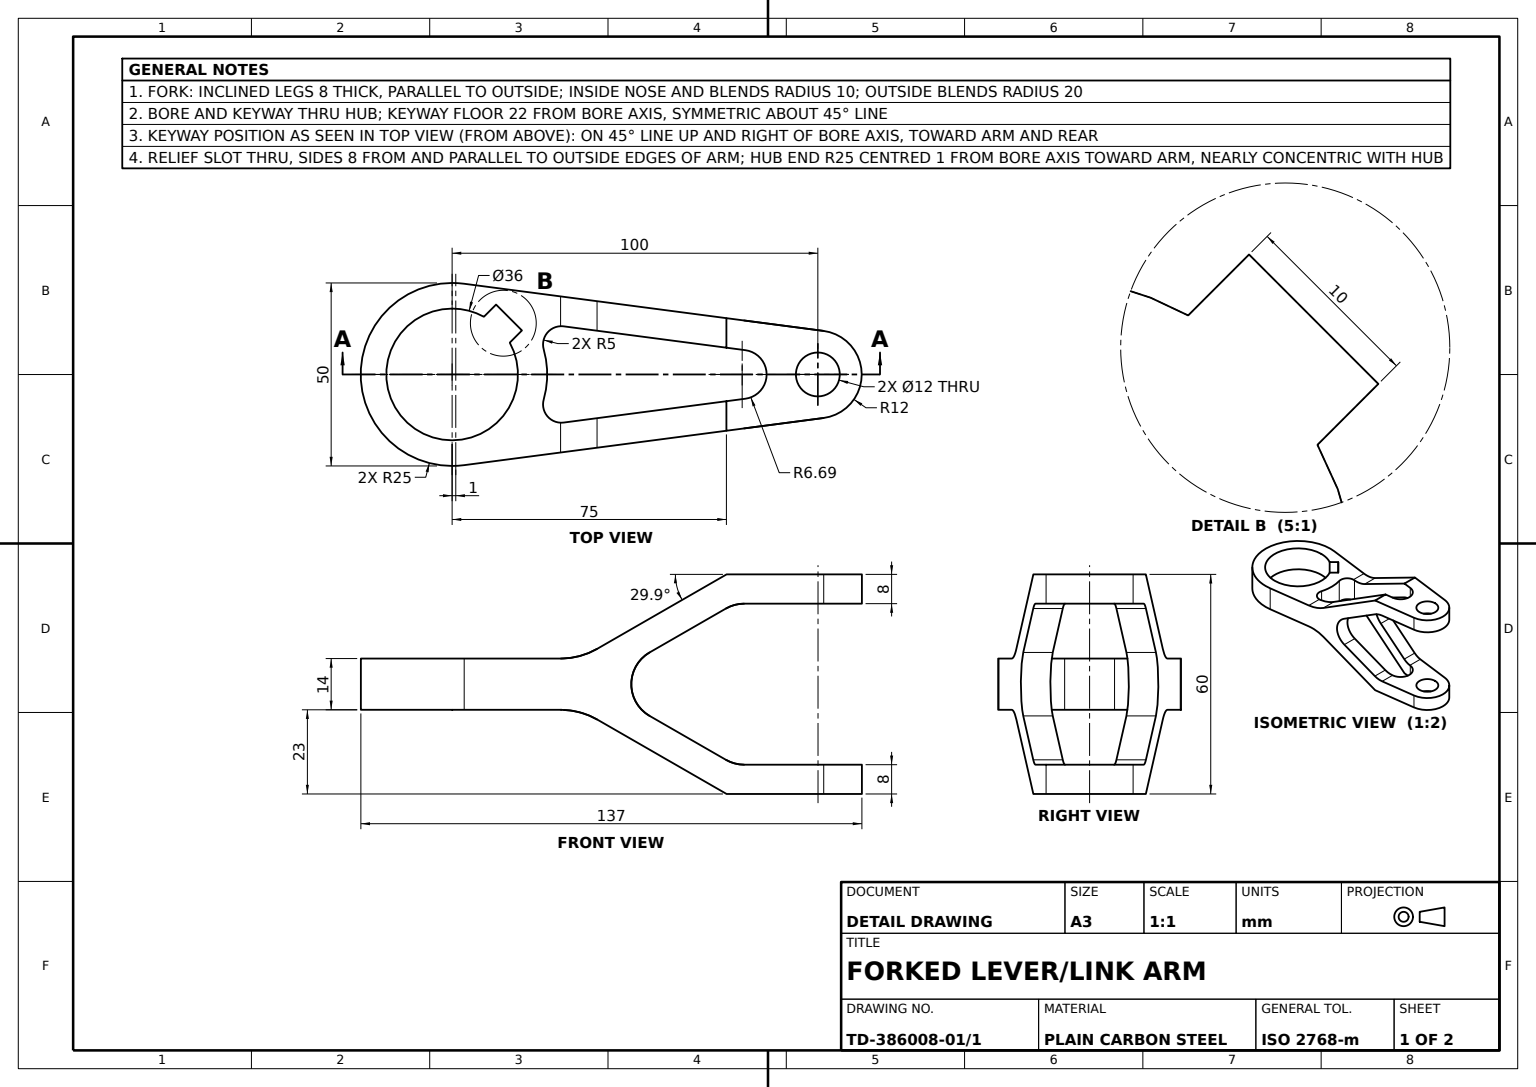
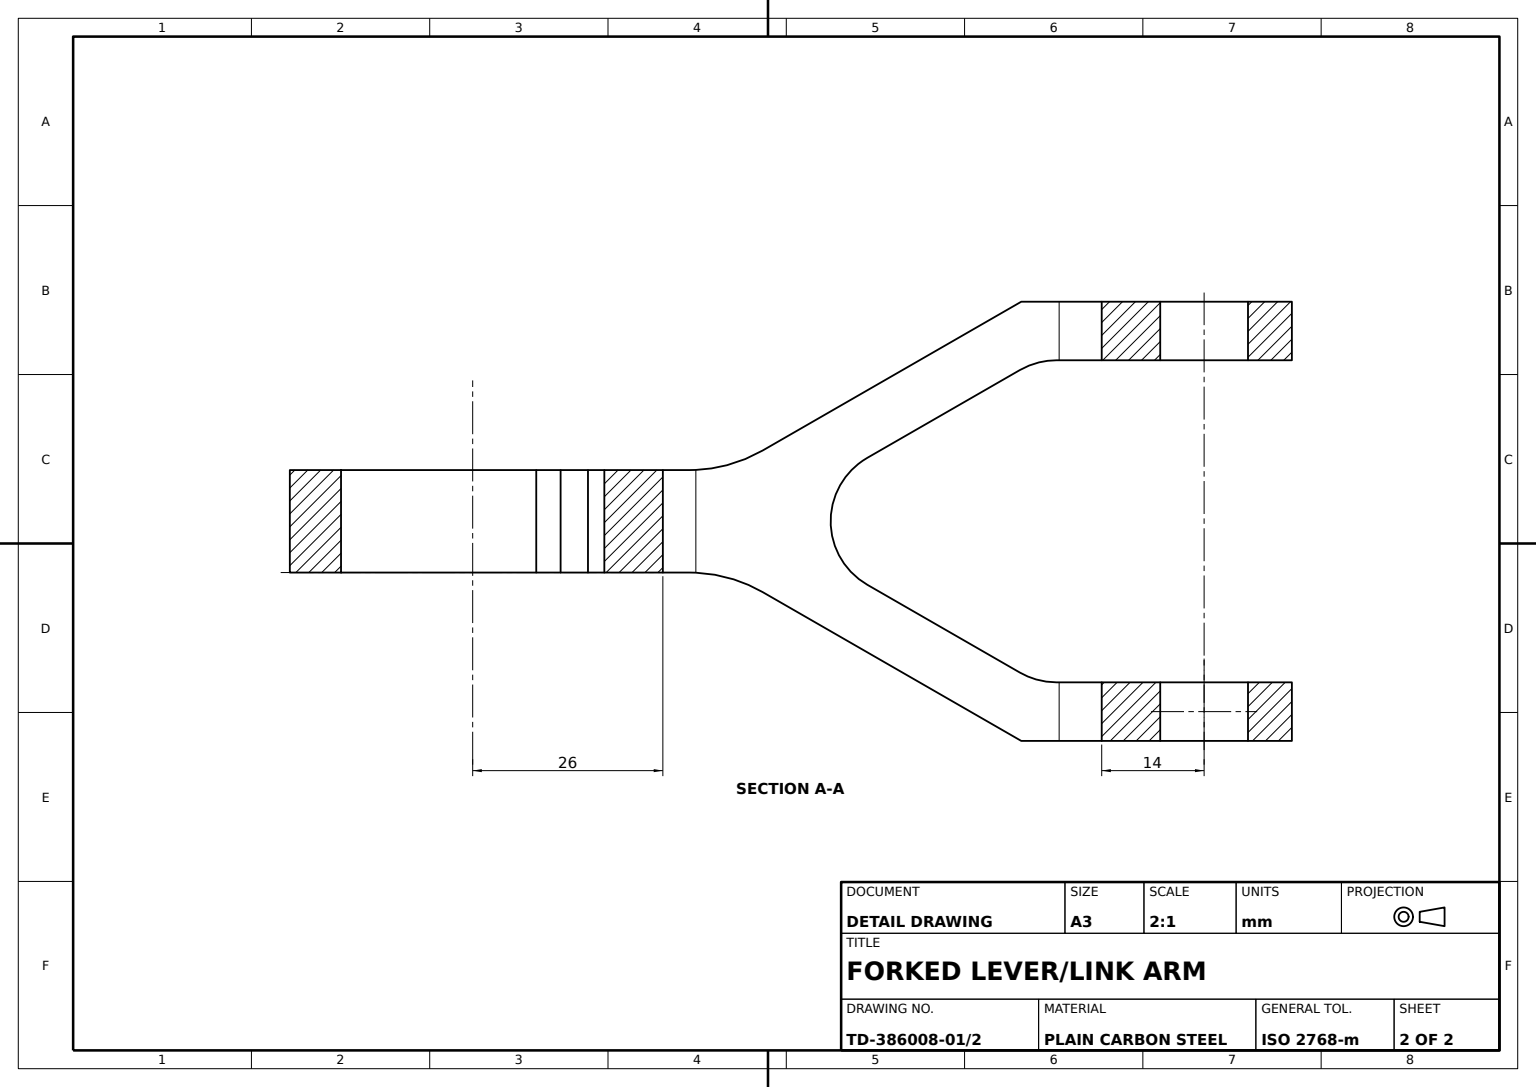
from build123d import *

# Parameters (mm, degrees)
LEVER_BLANK_DEPTH             = 30
HUB_BORE_36_WITH_KEYWAY_DEPTH = 100.247166206
HOLE_12_SKETCH_R              = 6
HOLE_12_DEPTH                 = 100.247166206
RELIEF_SLOT_DEPTH             = 100.247166206
FORK_OUTLINE_CUT_DEPTH        = 30
ARM_LIGHTENING_WINDOWS_DEPTH  = 30


with BuildPart() as part:
    # Side Profile Sketch → Lever Blank (new, symmetric)
    with BuildSketch(Plane(origin=(0, 0, 0), x_dir=(1, 0, 0), z_dir=(0, 1, 0))):
        with BuildLine():
            Line((-46.75, 24.787849846), (51.56, 11.898167926))
            ThreePointArc((51.56, 11.898167926), (62, 0), (51.56, -11.898167926))
            Line((51.56, -11.898167926), (-46.75, -24.787849846))
            ThreePointArc((-46.75, -24.787849846), (-75, 0), (-46.75, 24.787849846))
        make_face()
    extrude(amount=LEVER_BLANK_DEPTH, both=True)

    # Hub Bore Sketch → Hub Bore Ø36 with Keyway (cut, through all)
    with BuildSketch(Plane(origin=(0, 30, 0), x_dir=(1, 0, 0), z_dir=(0, 1, 0))):
        with BuildLine():
            Line((-41.308514645, 15.762553167), (-37.97918472, 19.091883092))
            Line((-37.97918472, 19.091883092), (-30.908116908, 12.02081528))
            Line((-30.908116908, 12.02081528), (-34.237446833, 8.691485355))
            ThreePointArc((-34.237446833, 8.691485355), (-62.727922061, -12.727922061), (-41.308514645, 15.762553167))
        make_face()
    extrude(amount=-HUB_BORE_36_WITH_KEYWAY_DEPTH, mode=Mode.SUBTRACT)

    # Hole Ø12 Sketch → Hole Ø12 (cut, through all)
    with BuildSketch(Plane(origin=(0, 30, 0), x_dir=(1, 0, 0), z_dir=(0, 1, 0))):
        with Locations(Location((50, 0, 0), (0, 0, 270))):
            Circle(HOLE_12_SKETCH_R)
    extrude(amount=-HOLE_12_DEPTH, mode=Mode.SUBTRACT)

    # Relief Slot Sketch → Relief Slot (cut, through all)
    with BuildSketch(Plane(origin=(0, 30, 0), x_dir=(1, 0, 0), z_dir=(0, 1, 0))):
        with BuildLine():
            Line((-19.488879252, 13.145103734), (30.18, 6.632886717))
            ThreePointArc((30.18, 6.632886717), (36, 0), (30.18, -6.632886717))
            Line((30.18, -6.632886717), (-19.488879252, -13.145103734))
            ThreePointArc((-19.488879252, -13.145103734), (-23.922952707, -11.455681264), (-24.949066043, -6.822944804))
            ThreePointArc((-24.949066043, -6.822944804), (-24, 0), (-24.949066043, 6.822944804))
            ThreePointArc((-24.949066043, 6.822944804), (-23.922952707, 11.455681264), (-19.488879252, 13.145103734))
        make_face()
    extrude(amount=-RELIEF_SLOT_DEPTH, mode=Mode.SUBTRACT)

    # Fork Outline Sketch → Fork Outline Cut (cut, symmetric)
    with BuildSketch(Plane.XY):
        with BuildLine():
            Line((-75, 30), (-75, 7))
            Line((-75, 7), (-20.340076505, 7))
            ThreePointArc((-20.340076505, 7), (-15.180741335, 7.676924142), (-10.370654019, 9.661873939))
            Line((-10.370654019, 9.661873939), (25, 30))
            Line((25, 30), (-75, 30))
        make_face()
        with BuildLine():
            Line((-75, -30), (-75, -7))
            Line((-75, -7), (-20.340076505, -7))
            ThreePointArc((-20.340076505, -7), (-15.180741335, -7.676924142), (-10.370654019, -9.661873939))
            Line((-10.370654019, -9.661873939), (25, -30))
            Line((25, -30), (-75, -30))
        make_face()
    extrude(amount=FORK_OUTLINE_CUT_DEPTH, both=True, mode=Mode.SUBTRACT)

    # Arm Windows Sketch → Arm Lightening Windows (cut, symmetric)
    with BuildSketch(Plane.XY):
        with BuildLine():
            Line((62, 22), (29.806068854, 22))
            ThreePointArc((29.806068854, 22), (27.226401269, 21.661537929), (24.821357612, 20.669063031))
            Line((24.821357612, 20.669063031), (3.951792394, 8.669063031))
            ThreePointArc((3.951792394, 8.669063031), (-1.063496363, 0), (3.951792394, -8.669063031))
            Line((3.951792394, -8.669063031), (24.821357612, -20.669063031))
            ThreePointArc((24.821357612, -20.669063031), (27.226401269, -21.661537929), (29.806068854, -22))
            Line((29.806068854, -22), (62, -22))
            Line((62, -22), (62, 22))
        make_face()
    extrude(amount=ARM_LIGHTENING_WINDOWS_DEPTH, both=True, mode=Mode.SUBTRACT)


solid = part.part
